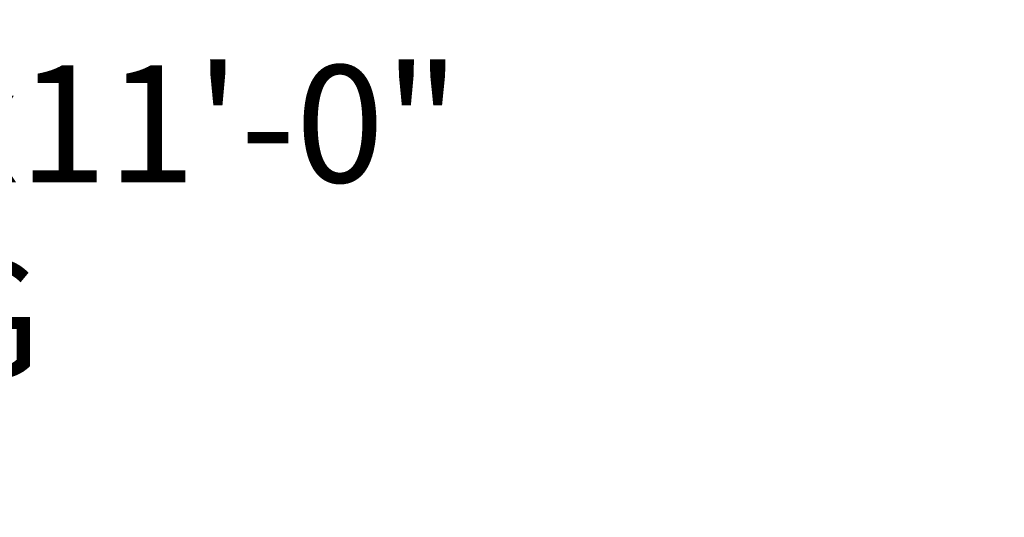
# Model space of a CAD drawing. Units: inches. Extents: x 2163 to 2982, y 1024 to 2288.
# Tile 15 of 22: x 2490 to 2532, y 1957 to 1978. Entities that reach past the tile are written whole.
import ezdxf

# ---------------------------------------------------------------- set-up
doc = ezdxf.new("R2010")
doc.units = ezdxf.units.IN
doc.layers.add('A-ANNO-DIMS', color=2, linetype='Continuous', lineweight=18)
doc.layers.add('A-AREA-IDEN', color=7, linetype='Continuous', lineweight=18)
doc.styles.get("Standard").update_dxf_attribs({"font": 'arial.ttf'})
doc.dimstyles.get("Standard").update_dxf_attribs({"dimtxt": 0.18, "dimasz": 0.18, "dimexe": 0.18, "dimexo": 0.0625, "dimgap": 0.09, "dimtad": 0, "dimtih": 1, "dimtoh": 1, "dimdec": 4, "dimzin": 0, "dimdsep": 46, "dimtxsty": 'Standard', "dimcen": 0.09, "dimadec": 0, "dimazin": 0, "dimtfac": 1, "dimtdec": 4, "dimtofl": 0, "dimtmove": 0, "dimatfit": 3, "dimfxl": 1, "dimtolj": 1, "dimtzin": 0, "dimarcsym": 0})

# ---------------------------------------------------------------- blocks, each defined once
blk = doc.blocks.new('*D29')
at = {"layer": 'A-ANNO-DIMS', "color": 0, "lineweight": -2, "transparency": 16777216}
for p, q in [((2285.339, 1738.831), (2285.339, 2288.099)), ((2867.339, 2229.331), (2867.339, 2288.099)), ((2285.519, 2287.919), (2576.051, 2287.919)), ((2867.159, 2287.919), (2576.627, 2287.919))]:
    blk.add_line(p, q, dxfattribs=at)
at = {"layer": 'A-ANNO-DIMS', "color": 0, "transparency": 16777216}
for points in [[(2285.519, 2287.949), (2285.519, 2287.889), (2285.339, 2287.919)], [(2867.159, 2287.949), (2867.159, 2287.889), (2867.339, 2287.919)]]:
    blk.add_solid(points, dxfattribs=at)
at = {"layer": 'Defpoints', "color": 0, "transparency": 16777216}
for p in [(2867.339, 2287.919), (2867.339, 2229.269), (2285.339, 1738.769)]:
    blk.add_point(p, dxfattribs=at)
at = {"layer": 'A-ANNO-DIMS', "color": 0, "transparency": 16777216, "insert": (2576.339, 2287.919), "char_height": 0.18, "attachment_point": 5}
blk.add_mtext('\\A1;582', dxfattribs=at)

msp = doc.modelspace()

# ---------------------------------------------------------------- texts
at = {"layer": 'A-AREA-IDEN', "insert": (2467.8359, 1976.1168), "char_height": 5, "attachment_point": 1}
msp.add_mtext_dynamic_manual_height_columns('11\'-0"x11\'-0"\\PDINING', width=71.336965, gutter_width=12.5, heights=[0], dxfattribs=at)

# ---------------------------------------------------------------- dimensions: what is measured, and where the dimension line sits
at = {"layer": 'A-ANNO-DIMS'}
dim = msp.add_linear_dim(base=(2867.3389, 2287.9188), p1=(2285.3389, 1738.7688), p2=(2867.3389, 2229.2688), dimstyle='Standard', override={"dimdec": 0, "dimlfac": 1, "dimrnd": 0, "dimzin": 0, "dimdsep": 46, "dimlunit": 2}, dxfattribs=at)
dim.commit()
dim.dimension.update_dxf_attribs({"geometry": '*D29', "text_midpoint": (2576.3389, 2287.9188)})

doc.saveas('drawing.dxf')
